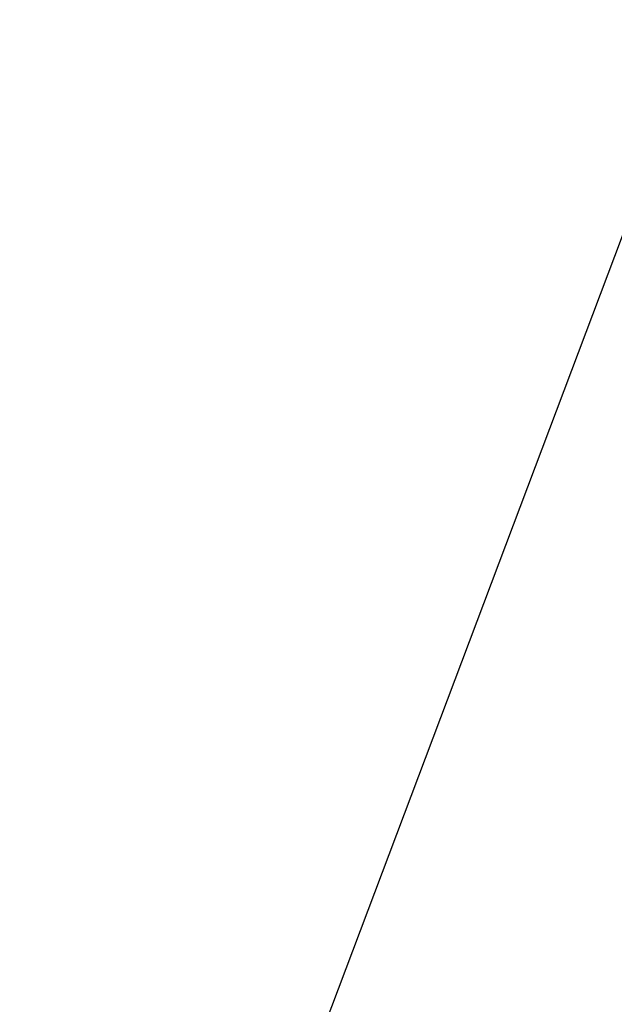
# Model space of a CAD drawing. Units: inches. Extents: x 3590 to 5167, y 65 to 1917.
# Tile 84 of 100: x 5051.5399 to 5051.6658, y 1788.6144 to 1788.8231. Entities that reach past the tile are written whole.
import ezdxf

# ---------------------------------------------------------------- set-up
doc = ezdxf.new("R2010")
doc.units = ezdxf.units.IN
for name, color, linetype, lineweight in [('A-ANNO-DIMS', 2, 'Continuous', 18), ('A-FLOR-PATT', 8, 'Continuous', 13), ('L-PLNT', 94, 'Continuous', 18)]:
    doc.layers.add(name, color=color, linetype=linetype, lineweight=lineweight)
doc.layers.add('DIENHOA', color=3, linetype='Continuous')
doc.styles.get("Standard").update_dxf_attribs({"font": 'arial.ttf'})
doc.dimstyles.new('ISO-25', dxfattribs={"dimtxt": 9, "dimasz": 2.5, "dimexe": 1.25, "dimexo": 0.625, "dimtad": 1, "dimdec": 1, "dimlunit": 3, "dimtxsty": 'Standard', "dimcen": 2.5, "dimadec": 0, "dimazin": 0, "dimtfac": 1, "dimtdec": 1, "dimtmove": 0, "dimatfit": 3, "dimfxl": 1, "dimarcsym": 0})

# ---------------------------------------------------------------- blocks, each defined once
blk = doc.blocks.new('Cay03_mb')
at = {"layer": 'DIENHOA'}
blk.add_lwpolyline([(23.6875, -5.4391), (19.839, 92.9868), (20.2832, 176.9678), (25.016, 248.5475), (34.0335, 309.7692), (47.3314, 362.6766), (64.9059, 409.3131), (86.7528, 451.7223), (112.868, 491.9476)], dxfattribs=at)
blk = doc.blocks.new('*D323')
at = {"layer": 'A-ANNO-DIMS', "color": 0, "lineweight": -2, "transparency": 16777216}
for p, q in [((5069.17227, 1795.21603), (5069.17227, 1874.95034)), ((5065.43703, 1795.21603), (5070.42227, 1795.21603)), ((5069.17227, 1769.30924), (5069.17227, 1792.71603)), ((5065.43703, 1766.80924), (5070.42227, 1766.80924))]:
    blk.add_line(p, q, dxfattribs=at)
at = {"layer": 'A-ANNO-DIMS', "color": 0, "transparency": 16777216}
for points in [[(5068.75561, 1792.71603), (5069.58894, 1792.71603), (5069.17227, 1795.21603)], [(5068.75561, 1769.30924), (5069.58894, 1769.30924), (5069.17227, 1766.80924)]]:
    blk.add_solid(points, dxfattribs=at)
at = {"layer": 'Defpoints', "color": 0, "transparency": 16777216}
for p in [(5064.81203, 1795.21603), (5069.17227, 1795.21603), (5064.81203, 1766.80924)]:
    blk.add_point(p, dxfattribs=at)
at = {"layer": 'A-ANNO-DIMS', "color": 0, "transparency": 16777216, "insert": (5063.89379, 1836.33318), "char_height": 9, "attachment_point": 5, "rotation": 90}
blk.add_mtext('2\'-4 1/2" TYP.', dxfattribs=at)

msp = doc.modelspace()

# ---------------------------------------------------------------- hatches: boundary and pattern name
at = {"layer": 'A-FLOR-PATT', "transparency": 33554687}
h = msp.add_hatch(dxfattribs=at)
h.set_pattern_fill('AR-HBONE', color=256, scale=0.2)
h.set_pattern_definition([(45, (-588.972, 0), (0, 28.73682), [60.96, -20.32]), (135, (-574.604, 14.368), (3e-15, 28.73682), [60.96, -20.32])])
h.paths.add_polyline_path([(5071.27403, 1796.99898), (4933.27403, 1796.99898), (4933.27403, 1753.99898), (4962.77403, 1753.99898, -0.414214), (4928.77403, 1719.99898), (4933.27403, 1718.99898), (4933.27403, 1334.99898), (5071.27403, 1334.99898)])
h.paths.add_polyline_path([(4951.78002, 1521.0767), (4951.7151, 1521.0404), (4951.56345, 1520.89532)], flags=16)
h.paths.add_polyline_path([(4952.267, 1521.37645), (4952.1977, 1521.37111), (4952.19823, 1521.35558)], flags=0)
h.paths.add_polyline_path([(4967.05076, 1529.72832), (4965.23122, 1528.69444), (4963.41109, 1527.71401), (4961.75649, 1526.85081), (4963.58887, 1527.44938), (4964.03555, 1527.47802), (4962.9755, 1527.24902), (4961.76022, 1526.85203), (4959.79219, 1525.83406), (4958.00498, 1524.89483), (4956.24031, 1523.92961), (4954.50395, 1522.91854), (4954.1294, 1522.68163), (4953.36051, 1521.99688), (4953.36558, 1521.99754), (4953.605, 1522.06367), (4955.10605, 1522.76083), (4956.92108, 1523.43405), (4958.67784, 1523.91513), (4960.35834, 1524.20036), (4961.94456, 1524.28606), (4964.17144, 1524.10849), (4965.95752, 1523.30903), (4963.86273, 1522.97565), (4965.18742, 1522.49898), (4963.36614, 1522.49715), (4961.54526, 1522.48682), (4959.76359, 1522.46077), (4958.30414, 1522.4188), (4957.97356, 1522.38829), (4956.30692, 1522.2324), (4954.71821, 1522.07143), (4953.25077, 1521.89915), (4953.52509, 1521.62277), (4954.33087, 1521.37883), (4956.24263, 1521.22987), (4958.03913, 1520.92952), (4959.68424, 1520.48339), (4961.16007, 1519.89569), (4963.10699, 1518.80022), (4964.39286, 1517.32518), (4962.97306, 1517.72596), (4964.55841, 1516.66059), (4965.40664, 1515.70779), (4963.50733, 1516.32179), (4961.67995, 1517.0051), (4959.93478, 1517.74489), (4958.2821, 1518.52833), (4956.73216, 1519.34257), (4955.29527, 1520.17478), (4954.67155, 1520.57237), (4954.51279, 1520.6271), (4955.65848, 1519.31837), (4956.70263, 1517.98232), (4957.64403, 1516.64663), (4958.48545, 1515.33439), (4959.54998, 1513.52398), (4960.43768, 1511.76936), (4958.84107, 1513.6196), (4957.45175, 1515.3249), (4955.8186, 1517.45855), (4956.66537, 1515.44764), (4957.11109, 1513.92292), (4957.44681, 1511.71434), (4957.07641, 1509.79288), (4956.53757, 1511.1103), (4955.99231, 1512.56892), (4955.44448, 1514.12509), (4954.89794, 1515.73518), (4954.35653, 1517.35553), (4953.82412, 1518.94251), (4953.30455, 1520.45247), (4953.06452, 1521.11563), (4952.97143, 1521.14607), (4952.94932, 1521.08646), (4952.72981, 1520.19905), (4953.3698, 1518.02364), (4953.75708, 1516.37279), (4954.05124, 1514.76538), (4954.26449, 1513.22121), (4954.47124, 1511.13121), (4954.4971, 1510.40174), (4954.40903, 1511.76006), (4954.26449, 1513.22121), (4954.05124, 1514.76538), (4953.75708, 1516.37279), (4953.3698, 1518.02364), (4952.87718, 1519.69813), (4952.7161, 1520.1412), (4952.53301, 1519.05871), (4952.37428, 1517.78881), (4952.21925, 1516.31167), (4952.04598, 1514.59986), (4951.83253, 1512.62598), (4951.55697, 1510.36259), (4951.20331, 1512.16818), (4950.85168, 1514.33931), (4950.98529, 1516.37594), (4951.6596, 1518.28625), (4952.59261, 1520.48085), (4952.35664, 1521.1299), (4951.85502, 1520.32753), (4950.83901, 1518.90828), (4949.77675, 1517.58658), (4948.91554, 1516.61731), (4948.11099, 1515.2561), (4947.0891, 1513.55389), (4945.88937, 1511.61495), (4946.32587, 1513.40232), (4946.5624, 1514.24913), (4945.52771, 1513.32668), (4944.58105, 1512.53126), (4946.01774, 1514.50825), (4947.2044, 1516.04763), (4947.89331, 1517.31331), (4949.30686, 1518.76446), (4950.41417, 1519.76716), (4950.45131, 1519.80628), (4952.267, 1521.37645), (4951.64457, 1521.49317), (4950.40371, 1521.17954), (4948.04447, 1520.35868), (4946.11863, 1519.45198), (4944.57182, 1518.47484), (4943.34962, 1517.44265), (4941.99695, 1515.91971), (4941.66146, 1515.27475), (4942.81332, 1516.98973), (4944.57182, 1518.47484), (4946.11863, 1519.45198), (4948.04447, 1520.35868), (4950.40371, 1521.17954), (4951.64457, 1521.49317), (4949.64678, 1521.86781), (4948.59979, 1521.75633), (4947.12629, 1521.5699), (4945.42015, 1521.34763), (4943.44969, 1521.10462), (4941.18319, 1520.85596), (4942.86028, 1521.61265), (4943.87308, 1522.03014), (4942.95216, 1521.9093), (4941.40968, 1521.48512), (4939.54287, 1520.67019), (4938.96775, 1520.2255), (4940.73284, 1521.29899), (4942.95216, 1521.9093), (4943.70184, 1522.00767), (4945.89419, 1522.69998), (4947.56488, 1522.71399), (4948.92086, 1522.56573), (4951.13144, 1522.18271), (4950.97062, 1522.2969), (4948.12924, 1523.00563), (4946.03496, 1523.70671), (4944.23235, 1524.52143), (4942.70692, 1525.46111), (4941.44419, 1526.53707), (4940.42968, 1527.76062), (4939.6489, 1529.14306), (4941.42091, 1528.12232), (4943.14742, 1527.13248), (4944.84093, 1526.17457), (4946.51394, 1525.24959), (4948.17893, 1524.35855), (4948.36457, 1524.26336), (4946.47531, 1526.04459), (4945.18083, 1527.54042), (4944.19039, 1529.03339), (4943.49559, 1530.53985), (4943.27808, 1531.3597), (4942.49849, 1531.91903), (4943.11353, 1531.76249), (4942.95927, 1533.6586), (4944.13953, 1531.9886), (4944.61171, 1531.32339), (4946.20163, 1530.46341), (4947.48567, 1529.50925), (4948.79027, 1528.22649), (4950.36754, 1526.23746), (4949.48547, 1528.15549), (4948.85128, 1530.12254), (4948.49054, 1532.04127), (4948.38105, 1533.91822), (4948.50062, 1535.7599), (4948.82704, 1537.57284), (4949.41803, 1535.56526), (4949.95684, 1533.56932), (4950.46414, 1531.5861), (4950.96058, 1529.6167), (4951.3911, 1527.95448), (4951.72352, 1530.68689), (4952.20106, 1532.57994), (4952.88914, 1534.32964), (4953.77035, 1535.95123), (4954.82726, 1537.45995), (4954.52145, 1535.38966), (4954.27314, 1533.93684), (4955.57999, 1535.6627), (4956.74758, 1536.73859), (4956.15852, 1534.78029), (4955.58917, 1532.87334), (4955.04336, 1531.00581), (4954.52493, 1529.16576), (4954.03771, 1527.34127), (4953.63833, 1525.73298), (4953.61143, 1525.58564), (4953.39805, 1524.16565), (4953.38219, 1524.00887), (4954.06955, 1525.47563), (4954.91212, 1527.02173), (4956.13627, 1528.89351), (4957.84668, 1530.57701), (4959.37601, 1531.54014), (4958.25596, 1530.10398), (4957.14284, 1528.66291), (4956.06626, 1527.24305), (4955.05579, 1525.87054), (4954.14104, 1524.57149), (4953.35159, 1523.37204), (4953.31079, 1523.30299), (4953.27253, 1522.92478), (4953.26102, 1522.38213), (4954.1031, 1523.37273), (4954.63005, 1524.28376), (4955.96149, 1526.35767), (4957.23002, 1528.12969), (4958.42057, 1529.60864), (4960.03671, 1531.36792), (4961.3736, 1532.3752), (4962.1015, 1532.77), (4961.06994, 1531.06113), (4959.98733, 1529.43811), (4958.86851, 1527.90803), (4958.15046, 1527.00742), (4959.80291, 1528.00314), (4961.58854, 1528.79257), (4963.39087, 1529.32783), (4965.21118, 1529.63205)], flags=16)
h.paths.add_polyline_path([(4962.94387, 1523.18187), (4961.10714, 1523.42192), (4960.39205, 1523.36158), (4962.34964, 1523.33061)], flags=0)
h.paths.add_polyline_path([(5049.54129, 1584.55089), (5049.47636, 1584.51458), (5049.32471, 1584.3695)], flags=16)
h.paths.add_polyline_path([(5050.02827, 1584.85063), (5049.95897, 1584.84529), (5049.95949, 1584.82976)], flags=0)
h.paths.add_polyline_path([(5042.33308, 1581.94902), (5043.8799, 1582.92616), (5045.80573, 1583.83286), (5048.16498, 1584.65372), (5049.40583, 1584.96736), (5047.40804, 1585.34199), (5046.36106, 1585.23052), (5044.88755, 1585.04408), (5043.18142, 1584.82181), (5041.21095, 1584.5788), (5038.94446, 1584.33014), (5040.62155, 1585.08683), (5041.63434, 1585.50432), (5040.71343, 1585.38348), (5039.17095, 1584.9593), (5037.30414, 1584.14438), (5036.72901, 1583.69969), (5038.4941, 1584.77317), (5040.71343, 1585.38348), (5041.4631, 1585.48185), (5043.65545, 1586.17416), (5045.32615, 1586.18818), (5046.68212, 1586.03992), (5048.8927, 1585.6569), (5048.73188, 1585.77108), (5045.89051, 1586.47981), (5043.79622, 1587.18089), (5041.99361, 1587.99561), (5040.46818, 1588.9353), (5039.20546, 1590.01125), (5038.19095, 1591.2348), (5037.41016, 1592.61725), (5039.18217, 1591.5965), (5040.90868, 1590.60667), (5042.6022, 1589.64876), (5044.2752, 1588.72378), (5045.94019, 1587.83274), (5046.12584, 1587.73754), (5044.23658, 1589.51878), (5042.9421, 1591.01461), (5041.95166, 1592.50757), (5041.25685, 1594.01403), (5041.03935, 1594.83388), (5040.25976, 1595.39321), (5040.8748, 1595.23667), (5040.72054, 1597.13279), (5041.9008, 1595.46278), (5042.37297, 1594.79758), (5043.96289, 1593.93759), (5045.24694, 1592.98344), (5046.55153, 1591.70068), (5048.12881, 1589.71164), (5047.24673, 1591.62967), (5046.61254, 1593.59672), (5046.2518, 1595.51546), (5046.14232, 1597.3924), (5046.26189, 1599.23408), (5046.5883, 1601.04703), (5047.17929, 1599.03944), (5047.71811, 1597.0435), (5048.22541, 1595.06028), (5048.72184, 1593.09089), (5049.15237, 1591.42866), (5049.48478, 1594.16107), (5049.96233, 1596.05412), (5050.65041, 1597.80382), (5051.53161, 1599.42541), (5052.58852, 1600.93414), (5052.28271, 1598.86384), (5052.03441, 1597.41102), (5053.34126, 1599.13689), (5054.50884, 1600.21277), (5053.91979, 1598.25447), (5053.35044, 1596.34752), (5052.80463, 1594.47999), (5052.2862, 1592.63995), (5051.79898, 1590.81546), (5051.39959, 1589.20716), (5051.3727, 1589.05983), (5051.15931, 1587.63984), (5051.14346, 1587.48305), (5051.83082, 1588.94982), (5052.67339, 1590.49592), (5053.89754, 1592.3677), (5055.60794, 1594.05119), (5057.13728, 1595.01432), (5056.01722, 1593.57817), (5054.90411, 1592.1371), (5053.82752, 1590.71724), (5052.81705, 1589.34472), (5051.9023, 1588.04567), (5051.11286, 1586.84622), (5051.07205, 1586.77718), (5051.03379, 1586.39896), (5051.02228, 1585.85631), (5051.86437, 1586.84692), (5052.39131, 1587.75794), (5053.72275, 1589.83185), (5054.99128, 1591.60387), (5056.18183, 1593.08282), (5057.79798, 1594.84211), (5059.13486, 1595.84938), (5059.86276, 1596.24419), (5058.83121, 1594.53531), (5057.7486, 1592.9123), (5056.62978, 1591.38221), (5055.91173, 1590.4816), (5057.56418, 1591.47732), (5059.34981, 1592.26675), (5061.15214, 1592.80202), (5062.97245, 1593.10624), (5064.81203, 1593.20251), (5062.99248, 1592.16863), (5061.17235, 1591.18819), (5059.51775, 1590.325), (5061.35014, 1590.92356), (5061.79682, 1590.95221), (5060.73676, 1590.7232), (5059.52148, 1590.32622), (5057.55345, 1589.30825), (5055.76625, 1588.36901), (5054.00157, 1587.40379), (5052.26521, 1586.39273), (5051.89067, 1586.15581), (5051.12177, 1585.47106), (5051.12684, 1585.47172), (5051.36627, 1585.53786), (5052.86732, 1586.23502), (5054.68234, 1586.90824), (5056.4391, 1587.38931), (5058.1196, 1587.67454), (5059.70582, 1587.76024), (5061.93271, 1587.58268), (5063.71878, 1586.78321), (5061.62399, 1586.44983), (5062.94869, 1585.97317), (5061.12741, 1585.97133), (5059.30653, 1585.961), (5057.52486, 1585.93496), (5056.06541, 1585.89299), (5055.73482, 1585.86247), (5054.06819, 1585.70658), (5052.47947, 1585.54561), (5051.01204, 1585.37333), (5051.28635, 1585.09695), (5052.09214, 1584.85301), (5054.00389, 1584.70406), (5055.8004, 1584.4037), (5057.44551, 1583.95757), (5058.92133, 1583.36987), (5060.86825, 1582.27441), (5062.15413, 1580.79937), (5060.73433, 1581.20015), (5062.31967, 1580.13477), (5063.1679, 1579.18198), (5061.2686, 1579.79597), (5059.44122, 1580.47928), (5057.69605, 1581.21908), (5056.04336, 1582.00251), (5054.49343, 1582.81675), (5053.05653, 1583.64897), (5052.43281, 1584.04656), (5052.27405, 1584.10128), (5053.41974, 1582.79255), (5054.4639, 1581.4565), (5055.40529, 1580.12081), (5056.24672, 1578.80858), (5057.31125, 1576.99816), (5058.19895, 1575.24354), (5056.60234, 1577.09378), (5055.21301, 1578.79908), (5053.57987, 1580.93274), (5054.42664, 1578.92183), (5054.87235, 1577.3971), (5055.20808, 1575.18852), (5054.83767, 1573.26706), (5054.29883, 1574.58448), (5053.75357, 1576.0431), (5053.20575, 1577.59927), (5052.6592, 1579.20936), (5052.1178, 1580.82971), (5051.58538, 1582.41669), (5051.06582, 1583.92666), (5050.82578, 1584.58981), (5050.7327, 1584.62025), (5050.71058, 1584.56064), (5050.49108, 1583.67323), (5051.13107, 1581.49782), (5051.51835, 1579.84698), (5051.8125, 1578.23957), (5052.02575, 1576.69539), (5052.23251, 1574.6054), (5052.25836, 1573.87593), (5052.1703, 1575.23424), (5052.02575, 1576.69539), (5051.8125, 1578.23957), (5051.51835, 1579.84698), (5051.13107, 1581.49782), (5050.63844, 1583.17231), (5050.47736, 1583.61538), (5050.29428, 1582.53289), (5050.13554, 1581.26299), (5049.98051, 1579.78585), (5049.80724, 1578.07405), (5049.59379, 1576.10016), (5049.31823, 1573.83678), (5048.96458, 1575.64237), (5048.61294, 1577.8135), (5048.74656, 1579.85012), (5049.42086, 1581.76043), (5050.35388, 1583.95503), (5050.1179, 1584.60408), (5049.61629, 1583.80172), (5048.60027, 1582.38246), (5047.53801, 1581.06076), (5046.67681, 1580.09149), (5045.87225, 1578.73029), (5044.85036, 1577.02808), (5043.65063, 1575.08913), (5044.08713, 1576.8765), (5044.32366, 1577.72331), (5043.28898, 1576.80086), (5042.34232, 1576.00545), (5043.779, 1577.98243), (5044.96566, 1579.52182), (5045.65457, 1580.78749), (5047.06813, 1582.23865), (5048.17543, 1583.24134), (5048.21258, 1583.28047), (5050.02827, 1584.85063), (5049.40583, 1584.96736), (5048.16498, 1584.65372), (5045.80573, 1583.83286), (5043.8799, 1582.92616), (5042.33308, 1581.94902), (5041.11088, 1580.91684), (5039.75821, 1579.39389), (5039.42272, 1578.74894), (5040.57458, 1580.46391)], flags=16)
h.paths.add_polyline_path([(4954.79872, 1533.12029), (4954.26249, 1532.07935), (4953.83112, 1530.93464), (4953.50472, 1529.63602), (4953.28338, 1528.13331), (4953.16721, 1526.37637), (4953.15631, 1524.31504), (4953.27669, 1521.23629), (4952.80168, 1521.84177), (4951.55695, 1521.99789), (4950.97575, 1521.9613), (4952.66059, 1521.94097), (4952.80168, 1521.84177), (4953.15249, 1523.59258), (4953.16721, 1526.37637), (4953.28338, 1528.13331), (4953.60929, 1530.34598), (4954.45558, 1532.59174)], flags=0)
h.paths.add_polyline_path([(5050.56294, 1585.31596), (5049.31822, 1585.47208), (5048.73702, 1585.43548), (5050.42186, 1585.41516), (5050.56294, 1585.31596), (5050.91375, 1587.06676), (5050.92848, 1589.85056), (5051.04465, 1591.6075), (5051.37055, 1593.82017), (5052.21684, 1596.06593), (5052.55999, 1596.59447), (5052.02375, 1595.55353), (5051.59238, 1594.40883), (5051.26598, 1593.1102), (5051.04465, 1591.6075), (5050.92848, 1589.85056), (5050.91757, 1587.78922), (5051.03795, 1584.71048)], flags=0)
h.paths.add_polyline_path([(5058.15332, 1586.83576), (5060.11091, 1586.80479), (5060.70514, 1586.65605), (5058.8684, 1586.8961)], flags=0)
h.paths.add_polyline_path([(5049.54129, 1430.93611), (5049.47636, 1430.8998), (5049.32471, 1430.75472)], flags=16)
h.paths.add_polyline_path([(5050.02827, 1431.23585), (5049.95897, 1431.23051), (5049.95949, 1431.21498)], flags=0)
h.paths.add_polyline_path([(5046.5883, 1447.43225), (5047.17929, 1445.42467), (5047.71811, 1443.42872), (5048.22541, 1441.4455), (5048.72184, 1439.47611), (5049.15237, 1437.81388), (5049.48478, 1440.5463), (5049.96233, 1442.43934), (5050.65041, 1444.18904), (5051.53161, 1445.81063), (5052.58852, 1447.31936), (5052.28271, 1445.24906), (5052.03441, 1443.79624), (5053.34126, 1445.52211), (5054.50884, 1446.59799), (5053.91979, 1444.63969), (5053.35044, 1442.73274), (5052.80463, 1440.86521), (5052.2862, 1439.02517), (5051.79898, 1437.20068), (5051.39959, 1435.59238), (5051.3727, 1435.44505), (5051.15931, 1434.02506), (5051.14346, 1433.86828), (5051.83082, 1435.33504), (5052.67339, 1436.88114), (5053.89754, 1438.75292), (5055.60794, 1440.43641), (5057.13728, 1441.39954), (5056.01722, 1439.96339), (5054.90411, 1438.52232), (5053.82752, 1437.10246), (5052.81705, 1435.72994), (5051.9023, 1434.4309), (5051.11286, 1433.23145), (5051.07205, 1433.1624), (5051.03379, 1432.78418), (5051.02228, 1432.24153), (5051.86437, 1433.23214), (5052.39131, 1434.14316), (5053.72275, 1436.21707), (5054.99128, 1437.98909), (5056.18183, 1439.46805), (5057.79798, 1441.22733), (5059.13486, 1442.23461), (5059.86276, 1442.62941), (5058.83121, 1440.92053), (5057.7486, 1439.29752), (5056.62978, 1437.76743), (5055.91173, 1436.86682), (5057.56418, 1437.86255), (5059.34981, 1438.65197), (5061.15214, 1439.18724), (5062.97245, 1439.49146), (5064.81203, 1439.58773), (5062.99248, 1438.55385), (5061.17235, 1437.57342), (5059.51775, 1436.71022), (5061.35014, 1437.30879), (5061.79682, 1437.33743), (5060.73676, 1437.10842), (5059.52148, 1436.71144), (5057.55345, 1435.69347), (5055.76625, 1434.75423), (5054.00157, 1433.78901), (5052.26521, 1432.77795), (5051.89067, 1432.54103), (5051.12177, 1431.85628), (5051.12684, 1431.85694), (5051.36627, 1431.92308), (5052.86732, 1432.62024), (5054.68234, 1433.29346), (5056.4391, 1433.77453), (5058.1196, 1434.05976), (5059.70582, 1434.14546), (5061.93271, 1433.9679), (5063.71878, 1433.16843), (5061.62399, 1432.83505), (5062.94869, 1432.35839), (5061.12741, 1432.35655), (5059.30653, 1432.34623), (5057.52486, 1432.32018), (5056.06541, 1432.27821), (5055.73482, 1432.24769), (5054.06819, 1432.09181), (5052.47947, 1431.93083), (5051.01204, 1431.75856), (5051.28635, 1431.48218), (5052.09214, 1431.23823), (5054.00389, 1431.08928), (5055.8004, 1430.78892), (5057.44551, 1430.34279), (5058.92133, 1429.75509), (5060.86825, 1428.65963), (5062.15413, 1427.18459), (5060.73433, 1427.58537), (5062.31967, 1426.52), (5063.1679, 1425.5672), (5061.2686, 1426.18119), (5059.44122, 1426.86451), (5057.69605, 1427.6043), (5056.04336, 1428.38773), (5054.49343, 1429.20197), (5053.05653, 1430.03419), (5052.43281, 1430.43178), (5052.27405, 1430.48651), (5053.41974, 1429.17777), (5054.4639, 1427.84172), (5055.40529, 1426.50603), (5056.24672, 1425.1938), (5057.31125, 1423.38338), (5058.19895, 1421.62877), (5056.60234, 1423.479), (5055.21301, 1425.1843), (5053.57987, 1427.31796), (5054.42664, 1425.30705), (5054.87235, 1423.78233), (5055.20808, 1421.57374), (5054.83767, 1419.65228), (5054.29883, 1420.9697), (5053.75357, 1422.42832), (5053.20575, 1423.9845), (5052.6592, 1425.59458), (5052.1178, 1427.21493), (5051.58538, 1428.80191), (5051.06582, 1430.31188), (5050.82578, 1430.97503), (5050.7327, 1431.00547), (5050.71058, 1430.94586), (5050.49108, 1430.05845), (5051.13107, 1427.88305), (5051.51835, 1426.2322), (5051.8125, 1424.62479), (5052.02575, 1423.08061), (5052.23251, 1420.99062), (5052.25836, 1420.26115), (5052.1703, 1421.61947), (5052.02575, 1423.08061), (5051.8125, 1424.62479), (5051.51835, 1426.2322), (5051.13107, 1427.88305), (5050.63844, 1429.55753), (5050.47736, 1430.0006), (5050.29428, 1428.91811), (5050.13554, 1427.64821), (5049.98051, 1426.17107), (5049.80724, 1424.45927), (5049.59379, 1422.48539), (5049.31823, 1420.222), (5048.96458, 1422.02759), (5048.61294, 1424.19872), (5048.74656, 1426.23534), (5049.42086, 1428.14565), (5050.35388, 1430.34025), (5050.1179, 1430.98931), (5049.61629, 1430.18694), (5048.60027, 1428.76768), (5047.53801, 1427.44598), (5046.67681, 1426.47671), (5045.87225, 1425.11551), (5044.85036, 1423.4133), (5043.65063, 1421.47435), (5044.08713, 1423.26172), (5044.32366, 1424.10854), (5043.28898, 1423.18608), (5042.34232, 1422.39067), (5043.779, 1424.36765), (5044.96566, 1425.90704), (5045.65457, 1427.17272), (5047.06813, 1428.62387), (5048.17543, 1429.62657), (5048.21258, 1429.66569), (5050.02827, 1431.23585), (5049.40583, 1431.35258), (5048.16498, 1431.03894), (5045.80573, 1430.21809), (5043.8799, 1429.31139), (5042.33308, 1428.33424), (5041.11088, 1427.30206), (5039.75821, 1425.77911), (5039.42272, 1425.13416), (5040.57458, 1426.84914), (5042.33308, 1428.33424), (5043.8799, 1429.31139), (5045.80573, 1430.21809), (5048.16498, 1431.03894), (5049.40583, 1431.35258), (5047.40804, 1431.72722), (5046.36106, 1431.61574), (5044.88755, 1431.42931), (5043.18142, 1431.20704), (5041.21095, 1430.96402), (5038.94446, 1430.71536), (5040.62155, 1431.47205), (5041.63434, 1431.88954), (5040.71343, 1431.76871), (5039.17095, 1431.34453), (5037.30414, 1430.5296), (5036.72901, 1430.08491), (5038.4941, 1431.1584), (5040.71343, 1431.76871), (5041.4631, 1431.86707), (5043.65545, 1432.55939), (5045.32615, 1432.5734), (5046.68212, 1432.42514), (5048.8927, 1432.04212), (5048.73188, 1432.1563), (5045.89051, 1432.86503), (5043.79622, 1433.56611), (5041.99361, 1434.38083), (5040.46818, 1435.32052), (5039.20546, 1436.39648), (5038.19095, 1437.62002), (5037.41016, 1439.00247), (5039.18217, 1437.98172), (5040.90868, 1436.99189), (5042.6022, 1436.03398), (5044.2752, 1435.109), (5045.94019, 1434.21796), (5046.12584, 1434.12276), (5044.23658, 1435.904), (5042.9421, 1437.39983), (5041.95166, 1438.8928), (5041.25685, 1440.39925), (5041.03935, 1441.2191), (5040.25976, 1441.77844), (5040.8748, 1441.62189), (5040.72054, 1443.51801), (5041.9008, 1441.848), (5042.37297, 1441.1828), (5043.96289, 1440.32282), (5045.24694, 1439.36866), (5046.55153, 1438.0859), (5048.12881, 1436.09686), (5047.24673, 1438.01489), (5046.61254, 1439.98195), (5046.2518, 1441.90068), (5046.14232, 1443.77762), (5046.26189, 1445.6193)], flags=16)
h.paths.add_polyline_path([(5052.38176, 1444.25496), (5051.62263, 1442.77987), (5052.02375, 1441.93875), (5052.55999, 1442.9797)], flags=0)
h.paths.add_polyline_path([(5050.56294, 1431.70118), (5049.31822, 1431.8573), (5048.73702, 1431.82071), (5050.42186, 1431.80038)], flags=0)
h.paths.add_polyline_path([(5058.15332, 1433.22098), (5060.11091, 1433.19001), (5060.70514, 1433.04127), (5058.8684, 1433.28132)], flags=0)
h.paths.add_polyline_path([(5049.54129, 1352.28535), (5049.47636, 1352.24904), (5049.32471, 1352.10396)], flags=16)
h.paths.add_polyline_path([(5050.02827, 1352.58509), (5049.95897, 1352.57975), (5049.95949, 1352.56422)], flags=0)
h.paths.add_polyline_path([(5046.5883, 1368.78149), (5047.17929, 1366.7739), (5047.71811, 1364.77796), (5048.22541, 1362.79474), (5048.72184, 1360.82534), (5049.15237, 1359.16312), (5049.48478, 1361.89553), (5049.96233, 1363.78858), (5050.65041, 1365.53828), (5051.53161, 1367.15987), (5052.58852, 1368.6686), (5052.28271, 1366.5983), (5052.03441, 1365.14548), (5053.34126, 1366.87135), (5054.50884, 1367.94723), (5053.91979, 1365.98893), (5053.35044, 1364.08198), (5052.80463, 1362.21445), (5052.2862, 1360.37441), (5051.79898, 1358.54992), (5051.39959, 1356.94162), (5051.3727, 1356.79428), (5051.15931, 1355.37429), (5051.14346, 1355.21751), (5051.83082, 1356.68428), (5052.67339, 1358.23037), (5053.89754, 1360.10216), (5055.60794, 1361.78565), (5057.13728, 1362.74878), (5056.01722, 1361.31262), (5054.90411, 1359.87155), (5053.82752, 1358.4517), (5052.81705, 1357.07918), (5051.9023, 1355.78013), (5051.11286, 1354.58068), (5051.07205, 1354.51164), (5051.03379, 1354.13342), (5051.02228, 1353.59077), (5051.86437, 1354.58137), (5052.39131, 1355.4924), (5053.72275, 1357.56631), (5054.99128, 1359.33833), (5056.18183, 1360.81728), (5057.79798, 1362.57656), (5059.13486, 1363.58384), (5059.86276, 1363.97864), (5058.83121, 1362.26977), (5057.7486, 1360.64675), (5056.62978, 1359.11667), (5055.91173, 1358.21606), (5057.56418, 1359.21178), (5059.34981, 1360.00121), (5061.15214, 1360.53648), (5062.97245, 1360.84069), (5064.81203, 1360.93697), (5062.99248, 1359.90308), (5061.17235, 1358.92265), (5059.51775, 1358.05946), (5061.35014, 1358.65802), (5061.79682, 1358.68666), (5060.73676, 1358.45766), (5059.52148, 1358.06068), (5057.55345, 1357.0427), (5055.76625, 1356.10347), (5054.00157, 1355.13825), (5052.26521, 1354.12718), (5051.89067, 1353.89027), (5051.12177, 1353.20552), (5051.12684, 1353.20618), (5051.36627, 1353.27231), (5052.86732, 1353.96947), (5054.68234, 1354.6427), (5056.4391, 1355.12377), (5058.1196, 1355.409), (5059.70582, 1355.4947), (5061.93271, 1355.31713), (5063.71878, 1354.51767), (5061.62399, 1354.18429), (5062.94869, 1353.70763), (5061.12741, 1353.70579), (5059.30653, 1353.69546), (5057.52486, 1353.66942), (5056.06541, 1353.62744), (5055.73482, 1353.59693), (5054.06819, 1353.44104), (5052.47947, 1353.28007), (5051.01204, 1353.10779), (5051.28635, 1352.83141), (5052.09214, 1352.58747), (5054.00389, 1352.43852), (5055.8004, 1352.13816), (5057.44551, 1351.69203), (5058.92133, 1351.10433), (5060.86825, 1350.00887), (5062.15413, 1348.53382), (5060.73433, 1348.9346), (5062.31967, 1347.86923), (5063.1679, 1346.91643), (5061.2686, 1347.53043), (5059.44122, 1348.21374), (5057.69605, 1348.95353), (5056.04336, 1349.73697), (5054.49343, 1350.55121), (5053.05653, 1351.38342), (5052.43281, 1351.78101), (5052.27405, 1351.83574), (5053.41974, 1350.52701), (5054.4639, 1349.19096), (5055.40529, 1347.85527), (5056.24672, 1346.54303), (5057.31125, 1344.73262), (5058.19895, 1342.978), (5056.60234, 1344.82824), (5055.21301, 1346.53354), (5053.57987, 1348.6672), (5054.42664, 1346.65629), (5054.87235, 1345.13156), (5055.20808, 1342.92298), (5054.83767, 1341.00152), (5054.29883, 1342.31894), (5053.75357, 1343.77756), (5053.20575, 1345.33373), (5052.6592, 1346.94382), (5052.1178, 1348.56417), (5051.58538, 1350.15115), (5051.06582, 1351.66111), (5050.82578, 1352.32427), (5050.7327, 1352.35471), (5050.71058, 1352.2951), (5050.49108, 1351.40769), (5051.13107, 1349.23228), (5051.51835, 1347.58144), (5051.8125, 1345.97403), (5052.02575, 1344.42985), (5052.23251, 1342.33986), (5052.25836, 1341.61039), (5052.1703, 1342.9687), (5052.02575, 1344.42985), (5051.8125, 1345.97403), (5051.51835, 1347.58144), (5051.13107, 1349.23228), (5050.63844, 1350.90677), (5050.47736, 1351.34984), (5050.29428, 1350.26735), (5050.13554, 1348.99745), (5049.98051, 1347.52031), (5049.80724, 1345.80851), (5049.59379, 1343.83462), (5049.31823, 1341.57124), (5048.96458, 1343.37683), (5048.61294, 1345.54796), (5048.74656, 1347.58458), (5049.42086, 1349.49489), (5050.35388, 1351.68949), (5050.1179, 1352.33854), (5049.61629, 1351.53617), (5048.60027, 1350.11692), (5047.53801, 1348.79522), (5046.67681, 1347.82595), (5045.87225, 1346.46475), (5044.85036, 1344.76253), (5043.65063, 1342.82359), (5044.08713, 1344.61096), (5044.32366, 1345.45777), (5043.28898, 1344.53532), (5042.34232, 1343.7399), (5043.779, 1345.71689), (5044.96566, 1347.25627), (5045.65457, 1348.52195), (5047.06813, 1349.9731), (5048.17543, 1350.9758), (5048.21258, 1351.01493), (5050.02827, 1352.58509), (5049.40583, 1352.70181), (5048.16498, 1352.38818), (5045.80573, 1351.56732), (5043.8799, 1350.66062), (5042.33308, 1349.68348), (5041.11088, 1348.65129), (5039.75821, 1347.12835), (5039.42272, 1346.4834), (5040.57458, 1348.19837), (5042.33308, 1349.68348), (5043.8799, 1350.66062), (5045.80573, 1351.56732), (5048.16498, 1352.38818), (5049.40583, 1352.70181), (5047.40804, 1353.07645), (5046.36106, 1352.96498), (5044.88755, 1352.77854), (5043.18142, 1352.55627), (5041.21095, 1352.31326), (5038.94446, 1352.0646), (5040.62155, 1352.82129), (5041.63434, 1353.23878), (5040.71343, 1353.11794), (5039.17095, 1352.69376), (5037.30414, 1351.87884), (5036.72901, 1351.43415), (5038.4941, 1352.50763), (5040.71343, 1353.11794), (5041.4631, 1353.21631), (5043.65545, 1353.90862), (5045.32615, 1353.92263), (5046.68212, 1353.77438), (5048.8927, 1353.39136), (5048.73188, 1353.50554), (5045.89051, 1354.21427), (5043.79622, 1354.91535), (5041.99361, 1355.73007), (5040.46818, 1356.66975), (5039.20546, 1357.74571), (5038.19095, 1358.96926), (5037.41016, 1360.35171), (5039.18217, 1359.33096), (5040.90868, 1358.34112), (5042.6022, 1357.38321), (5044.2752, 1356.45824), (5045.94019, 1355.5672), (5046.12584, 1355.472), (5044.23658, 1357.25323), (5042.9421, 1358.74906), (5041.95166, 1360.24203), (5041.25685, 1361.74849), (5041.03935, 1362.56834), (5040.25976, 1363.12767), (5040.8748, 1362.97113), (5040.72054, 1364.86725), (5041.9008, 1363.19724), (5042.37297, 1362.53203), (5043.96289, 1361.67205), (5045.24694, 1360.7179), (5046.55153, 1359.43513), (5048.12881, 1357.4461), (5047.24673, 1359.36413), (5046.61254, 1361.33118), (5046.2518, 1363.24992), (5046.14232, 1365.12686), (5046.26189, 1366.96854)], flags=16)
h.paths.add_polyline_path([(5052.38176, 1365.6042), (5051.62263, 1364.12911), (5052.02375, 1363.28799), (5052.55999, 1364.32893)], flags=0)
h.paths.add_polyline_path([(4951.78002, 1698.04081), (4951.7151, 1698.0045), (4951.56345, 1697.85942)], flags=16)
h.paths.add_polyline_path([(4952.267, 1698.34055), (4952.1977, 1698.33521), (4952.19823, 1698.31968)], flags=0)
h.paths.add_polyline_path([(4957.07641, 1686.75698), (4956.53757, 1688.0744), (4955.99231, 1689.53302), (4955.44448, 1691.08919), (4954.89794, 1692.69928), (4954.35653, 1694.31963), (4953.82412, 1695.90661), (4953.30455, 1697.41658), (4953.06452, 1698.07973), (4952.97143, 1698.11017), (4952.94932, 1698.05056), (4952.72981, 1697.16315), (4953.3698, 1694.98774), (4953.75708, 1693.3369), (4954.05124, 1691.72949), (4954.26449, 1690.18531), (4954.47124, 1688.09532), (4954.4971, 1687.36585), (4954.40903, 1688.72416), (4954.26449, 1690.18531), (4954.05124, 1691.72949), (4953.75708, 1693.3369), (4953.3698, 1694.98774), (4952.87718, 1696.66223), (4952.7161, 1697.1053), (4952.53301, 1696.02281), (4952.37428, 1694.75291), (4952.21925, 1693.27577), (4952.04598, 1691.56397), (4951.83253, 1689.59008), (4951.55697, 1687.3267), (4951.20331, 1689.13229), (4950.85168, 1691.30342), (4950.98529, 1693.34004), (4951.6596, 1695.25035), (4952.59261, 1697.44495), (4952.35664, 1698.09401), (4951.85502, 1697.29164), (4950.83901, 1695.87238), (4949.77675, 1694.55068), (4948.91554, 1693.58141), (4948.11099, 1692.22021), (4947.0891, 1690.518), (4945.88937, 1688.57905), (4946.32587, 1690.36642), (4946.5624, 1691.21323), (4945.52771, 1690.29078), (4944.58105, 1689.49537), (4946.01774, 1691.47235), (4947.2044, 1693.01174), (4947.89331, 1694.27741), (4949.30686, 1695.72857), (4950.41417, 1696.73127), (4950.45131, 1696.77039), (4952.267, 1698.34055), (4951.64457, 1698.45728), (4950.40371, 1698.14364), (4948.04447, 1697.32278), (4946.11863, 1696.41608), (4944.57182, 1695.43894), (4943.34962, 1694.40676), (4941.99695, 1692.88381), (4941.66146, 1692.23886), (4942.81332, 1693.95383), (4944.57182, 1695.43894), (4946.11863, 1696.41608), (4948.04447, 1697.32278), (4950.40371, 1698.14364), (4951.64457, 1698.45728), (4949.64678, 1698.83191), (4948.59979, 1698.72044), (4947.12629, 1698.53401), (4945.42015, 1698.31174), (4943.44969, 1698.06872), (4941.18319, 1697.82006), (4942.86028, 1698.57675), (4943.87308, 1698.99424), (4942.95216, 1698.8734), (4941.40968, 1698.44922), (4939.54287, 1697.6343), (4938.96775, 1697.18961), (4940.73284, 1698.26309), (4942.95216, 1698.8734), (4943.70184, 1698.97177), (4945.89419, 1699.66409), (4947.56488, 1699.6781), (4948.92086, 1699.52984), (4951.13144, 1699.14682), (4950.97062, 1699.261), (4948.12924, 1699.96973), (4946.03496, 1700.67081), (4944.23235, 1701.48553), (4942.70692, 1702.42522), (4941.44419, 1703.50117), (4940.42968, 1704.72472), (4939.6489, 1706.10717), (4941.42091, 1705.08642), (4943.14742, 1704.09659), (4944.84093, 1703.13868), (4946.51394, 1702.2137), (4948.17893, 1701.32266), (4948.36457, 1701.22746), (4946.47531, 1703.0087), (4945.18083, 1704.50453), (4944.19039, 1705.9975), (4943.49559, 1707.50395), (4943.27808, 1708.3238), (4942.49849, 1708.88314), (4943.11353, 1708.72659), (4942.95927, 1710.62271), (4944.13953, 1708.9527), (4944.61171, 1708.2875), (4946.20163, 1707.42751), (4947.48567, 1706.47336), (4948.79027, 1705.1906), (4950.36754, 1703.20156), (4949.48547, 1705.11959), (4948.85128, 1707.08664), (4948.49054, 1709.00538), (4948.38105, 1710.88232), (4948.50062, 1712.724), (4948.82704, 1714.53695), (4949.41803, 1712.52937), (4949.95684, 1710.53342), (4950.46414, 1708.5502), (4950.96058, 1706.58081), (4951.3911, 1704.91858), (4951.72352, 1707.65099), (4952.20106, 1709.54404), (4952.88914, 1711.29374), (4953.77035, 1712.91533), (4954.82726, 1714.42406), (4954.52145, 1712.35376), (4954.27314, 1710.90094), (4955.57999, 1712.62681), (4956.74758, 1713.70269), (4956.15852, 1711.74439), (4955.58917, 1709.83744), (4955.04336, 1707.96991), (4954.52493, 1706.12987), (4954.03771, 1704.30538), (4953.63833, 1702.69708), (4953.61143, 1702.54975), (4953.39805, 1701.12976), (4953.38219, 1700.97297), (4954.06955, 1702.43974), (4954.91212, 1703.98584), (4956.13627, 1705.85762), (4957.84668, 1707.54111), (4959.37601, 1708.50424), (4958.25596, 1707.06809), (4957.14284, 1705.62702), (4956.06626, 1704.20716), (4955.05579, 1702.83464), (4954.14104, 1701.53559), (4953.35159, 1700.33614), (4953.31079, 1700.2671), (4953.27253, 1699.88888), (4953.26102, 1699.34623), (4954.1031, 1700.33684), (4954.63005, 1701.24786), (4955.96149, 1703.32177), (4957.23002, 1705.09379), (4958.42057, 1706.57274), (4960.03671, 1708.33203), (4961.3736, 1709.33931), (4962.1015, 1709.73411), (4961.06994, 1708.02523), (4959.98733, 1706.40222), (4958.86851, 1704.87213), (4958.15046, 1703.97152), (4959.80291, 1704.96725), (4961.58854, 1705.75667), (4963.39087, 1706.29194), (4965.21118, 1706.59616), (4967.05076, 1706.69243), (4965.23122, 1705.65855), (4963.41109, 1704.67811), (4961.75649, 1703.81492), (4963.58887, 1704.41349), (4964.03555, 1704.44213), (4962.9755, 1704.21312), (4961.76022, 1703.81614), (4959.79219, 1702.79817), (4958.00498, 1701.85893), (4956.24031, 1700.89371), (4954.50395, 1699.88265), (4954.1294, 1699.64573), (4953.36051, 1698.96098), (4953.36558, 1698.96164), (4953.605, 1699.02778), (4955.10605, 1699.72494), (4956.92108, 1700.39816), (4958.67784, 1700.87923), (4960.35834, 1701.16446), (4961.94456, 1701.25016), (4964.17144, 1701.0726), (4965.95752, 1700.27313), (4963.86273, 1699.93975), (4965.18742, 1699.46309), (4963.36614, 1699.46125), (4961.54526, 1699.45092), (4959.76359, 1699.42488), (4958.30414, 1699.38291), (4957.97356, 1699.35239), (4956.30692, 1699.1965), (4954.71821, 1699.03553), (4953.25077, 1698.86326), (4953.52509, 1698.58688), (4954.33087, 1698.34293), (4956.24263, 1698.19398), (4958.03913, 1697.89362), (4959.68424, 1697.44749), (4961.16007, 1696.85979), (4963.10699, 1695.76433), (4964.39286, 1694.28929), (4962.97306, 1694.69007), (4964.55841, 1693.6247), (4965.40664, 1692.6719), (4963.50733, 1693.28589), (4961.67995, 1693.9692), (4959.93478, 1694.709), (4958.2821, 1695.49243), (4956.73216, 1696.30667), (4955.29527, 1697.13889), (4954.67155, 1697.53648), (4954.51279, 1697.5912), (4955.65848, 1696.28247), (4956.70263, 1694.94642), (4957.64403, 1693.61073), (4958.48545, 1692.2985), (4959.54998, 1690.48808), (4960.43768, 1688.73346), (4958.84107, 1690.5837), (4957.45175, 1692.289), (4955.8186, 1694.42266), (4956.66537, 1692.41175), (4957.11109, 1690.88702), (4957.44681, 1688.67844)], flags=16)
h.paths.add_polyline_path([(5050.56294, 1353.05042), (5049.31822, 1353.20654), (5048.73702, 1353.16994), (5050.42186, 1353.14961)], flags=0)
h.paths.add_polyline_path([(4951.78002, 1351.48609), (4951.7151, 1351.44979), (4951.56345, 1351.30471)], flags=16)
h.paths.add_polyline_path([(4952.267, 1351.78584), (4952.1977, 1351.7805), (4952.19823, 1351.76497)], flags=0)
h.paths.add_polyline_path([(4954.82726, 1367.86934), (4954.52145, 1365.79905), (4954.27314, 1364.34623), (4955.57999, 1366.07209), (4956.74758, 1367.14798), (4956.15852, 1365.18968), (4955.58917, 1363.28273), (4955.04336, 1361.4152), (4954.52493, 1359.57515), (4954.03771, 1357.75066), (4953.63833, 1356.14237), (4953.61143, 1355.99503), (4953.39805, 1354.57504), (4953.38219, 1354.41826), (4954.06955, 1355.88503), (4954.91212, 1357.43112), (4956.13627, 1359.3029), (4957.84668, 1360.9864), (4959.37601, 1361.94953), (4958.25596, 1360.51337), (4957.14284, 1359.0723), (4956.06626, 1357.65245), (4955.05579, 1356.27993), (4954.14104, 1354.98088), (4953.35159, 1353.78143), (4953.31079, 1353.71238), (4953.27253, 1353.33417), (4953.26102, 1352.79152), (4954.1031, 1353.78212), (4954.63005, 1354.69315), (4955.96149, 1356.76706), (4957.23002, 1358.53908), (4958.42057, 1360.01803), (4960.03671, 1361.77731), (4961.3736, 1362.78459), (4962.1015, 1363.17939), (4961.06994, 1361.47052), (4959.98733, 1359.8475), (4958.86851, 1358.31742), (4958.15046, 1357.41681), (4959.80291, 1358.41253), (4961.58854, 1359.20196), (4963.39087, 1359.73723), (4965.21118, 1360.04144), (4967.05076, 1360.13771), (4965.23122, 1359.10383), (4963.41109, 1358.1234), (4961.75649, 1357.26021), (4963.58887, 1357.85877), (4964.03555, 1357.88741), (4962.9755, 1357.65841), (4961.76022, 1357.26143), (4959.79219, 1356.24345), (4958.00498, 1355.30422), (4956.24031, 1354.339), (4954.50395, 1353.32793), (4954.1294, 1353.09102), (4953.36051, 1352.40627), (4953.36558, 1352.40693), (4953.605, 1352.47306), (4955.10605, 1353.17022), (4956.92108, 1353.84345), (4958.67784, 1354.32452), (4960.35834, 1354.60975), (4961.94456, 1354.69545), (4964.17144, 1354.51788), (4965.95752, 1353.71842), (4963.86273, 1353.38504), (4965.18742, 1352.90838), (4963.36614, 1352.90654), (4961.54526, 1352.89621), (4959.76359, 1352.87016), (4958.30414, 1352.82819), (4957.97356, 1352.79768), (4956.30692, 1352.64179), (4954.71821, 1352.48082), (4953.25077, 1352.30854), (4953.52509, 1352.03216), (4954.33087, 1351.78822), (4956.24263, 1351.63926), (4958.03913, 1351.33891), (4959.68424, 1350.89278), (4961.16007, 1350.30508), (4963.10699, 1349.20961), (4964.39286, 1347.73457), (4962.97306, 1348.13535), (4964.55841, 1347.06998), (4965.40664, 1346.11718), (4963.50733, 1346.73118), (4961.67995, 1347.41449), (4959.93478, 1348.15428), (4958.2821, 1348.93772), (4956.73216, 1349.75196), (4955.29527, 1350.58417), (4954.67155, 1350.98176), (4954.51279, 1351.03649), (4955.65848, 1349.72776), (4956.70263, 1348.39171), (4957.64403, 1347.05602), (4958.48545, 1345.74378), (4959.54998, 1343.93337), (4960.43768, 1342.17875), (4958.84107, 1344.02899), (4957.45175, 1345.73429), (4955.8186, 1347.86795), (4956.66537, 1345.85703), (4957.11109, 1344.33231), (4957.44681, 1342.12373), (4957.07641, 1340.20227), (4956.53757, 1341.51969), (4955.99231, 1342.97831), (4955.44448, 1344.53448), (4954.89794, 1346.14457), (4954.35653, 1347.76492), (4953.82412, 1349.3519), (4953.30455, 1350.86186), (4953.06452, 1351.52502), (4952.97143, 1351.55546), (4952.94932, 1351.49585), (4952.72981, 1350.60844), (4953.3698, 1348.43303), (4953.75708, 1346.78218), (4954.05124, 1345.17477), (4954.26449, 1343.6306), (4954.47124, 1341.5406), (4954.4971, 1340.81113), (4954.40903, 1342.16945), (4954.26449, 1343.6306), (4954.05124, 1345.17477), (4953.75708, 1346.78218), (4953.3698, 1348.43303), (4952.87718, 1350.10752), (4952.7161, 1350.55059), (4952.53301, 1349.4681), (4952.37428, 1348.1982), (4952.21925, 1346.72106), (4952.04598, 1345.00926), (4951.83253, 1343.03537), (4951.55697, 1340.77198), (4951.20331, 1342.57757), (4950.85168, 1344.7487), (4950.98529, 1346.78533), (4951.6596, 1348.69564), (4952.59261, 1350.89024), (4952.35664, 1351.53929), (4951.85502, 1350.73692), (4950.83901, 1349.31767), (4949.77675, 1347.99597), (4948.91554, 1347.0267), (4948.11099, 1345.66549), (4947.0891, 1343.96328), (4945.88937, 1342.02434), (4946.32587, 1343.81171), (4946.5624, 1344.65852), (4945.52771, 1343.73607), (4944.58105, 1342.94065), (4946.01774, 1344.91764), (4947.2044, 1346.45702), (4947.89331, 1347.7227), (4949.30686, 1349.17385), (4950.41417, 1350.17655), (4950.45131, 1350.21567), (4952.267, 1351.78584), (4951.64457, 1351.90256), (4950.40371, 1351.58893), (4948.04447, 1350.76807), (4946.11863, 1349.86137), (4944.57182, 1348.88423), (4943.34962, 1347.85204), (4941.99695, 1346.3291), (4941.66146, 1345.68414), (4942.81332, 1347.39912), (4944.57182, 1348.88423), (4946.11863, 1349.86137), (4948.04447, 1350.76807), (4950.40371, 1351.58893), (4951.64457, 1351.90256), (4949.64678, 1352.2772), (4948.59979, 1352.16572), (4947.12629, 1351.97929), (4945.42015, 1351.75702), (4943.44969, 1351.51401), (4941.18319, 1351.26535), (4942.86028, 1352.02204), (4943.87308, 1352.43953), (4942.95216, 1352.31869), (4941.40968, 1351.89451), (4939.54287, 1351.07958), (4938.96775, 1350.63489), (4940.73284, 1351.70838), (4942.95216, 1352.31869), (4943.70184, 1352.41706), (4945.89419, 1353.10937), (4947.56488, 1353.12338), (4948.92086, 1352.97513), (4951.13144, 1352.59211), (4950.97062, 1352.70629), (4948.12924, 1353.41502), (4946.03496, 1354.1161), (4944.23235, 1354.93082), (4942.70692, 1355.8705), (4941.44419, 1356.94646), (4940.42968, 1358.17001), (4939.6489, 1359.55246), (4941.42091, 1358.53171), (4943.14742, 1357.54187), (4944.84093, 1356.58396), (4946.51394, 1355.65898), (4948.17893, 1354.76794), (4948.36457, 1354.67275), (4946.47531, 1356.45398), (4945.18083, 1357.94981), (4944.19039, 1359.44278), (4943.49559, 1360.94924), (4943.27808, 1361.76909), (4942.49849, 1362.32842), (4943.11353, 1362.17188), (4942.95927, 1364.06799), (4944.13953, 1362.39799), (4944.61171, 1361.73278), (4946.20163, 1360.8728), (4947.48567, 1359.91864), (4948.79027, 1358.63588), (4950.36754, 1356.64685), (4949.48547, 1358.56488), (4948.85128, 1360.53193), (4948.49054, 1362.45066), (4948.38105, 1364.32761), (4948.50062, 1366.16929), (4948.82704, 1367.98223), (4949.41803, 1365.97465), (4949.95684, 1363.97871), (4950.46414, 1361.99549), (4950.96058, 1360.02609), (4951.3911, 1358.36387), (4951.72352, 1361.09628), (4952.20106, 1362.98933), (4952.88914, 1364.73903), (4953.77035, 1366.36062)], flags=16)
h.paths.add_polyline_path([(4954.79872, 1363.52968), (4954.26249, 1362.48874), (4953.83112, 1361.34403), (4953.50472, 1360.04541), (4953.28338, 1358.54271), (4953.16721, 1356.78577), (4953.15631, 1354.72443), (4953.27669, 1351.64568), (4952.80168, 1352.25116), (4951.55695, 1352.40728), (4950.97575, 1352.37069), (4952.66059, 1352.35036), (4952.80168, 1352.25116), (4953.15249, 1354.00197), (4953.16721, 1356.78577), (4953.28338, 1358.54271), (4953.60929, 1360.75537), (4954.45558, 1363.00113)], flags=0)
h.paths.add_polyline_path([(4952.80168, 1698.80588), (4951.55695, 1698.962), (4950.97575, 1698.92541), (4952.66059, 1698.90508), (4952.80168, 1698.80588), (4953.15249, 1700.55668), (4953.16721, 1703.34048), (4953.28338, 1705.09742), (4953.60929, 1707.31009), (4954.45558, 1709.55585), (4954.79872, 1710.0844), (4954.26249, 1709.04345), (4953.83112, 1707.89875), (4953.50472, 1706.60012), (4953.28338, 1705.09742), (4953.16721, 1703.34048), (4953.15631, 1701.27914), (4953.27669, 1698.2004)], flags=0)
h.paths.add_polyline_path([(4962.94387, 1700.14597), (4961.10714, 1700.38602), (4960.39205, 1700.32568), (4962.34964, 1700.29471)], flags=0)
h.paths.add_polyline_path([(5058.15332, 1354.57022), (5060.11091, 1354.53925), (5060.70514, 1354.39051), (5058.8684, 1354.63056)], flags=0)
h.paths.add_polyline_path([(4962.94387, 1353.59126), (4961.10714, 1353.83131), (4960.39205, 1353.77097), (4962.34964, 1353.74)], flags=0)
h.paths.add_polyline_path([(5049.54129, 1778.71989), (5049.47636, 1778.68358), (5049.32471, 1778.5385)], flags=16)
h.paths.add_polyline_path([(5050.02827, 1779.01963), (5049.95897, 1779.01429), (5049.95949, 1778.99876)], flags=0)
h.paths.add_polyline_path([(5052.25836, 1768.04493), (5052.1703, 1769.40324), (5052.02575, 1770.86439), (5051.8125, 1772.40857), (5051.51835, 1774.01598), (5051.13107, 1775.66682), (5050.63844, 1777.34131), (5050.47736, 1777.78438), (5050.29428, 1776.70189), (5050.13554, 1775.43199), (5049.98051, 1773.95485), (5049.80724, 1772.24305), (5049.59379, 1770.26916), (5049.31823, 1768.00578), (5048.96458, 1769.81137), (5048.61294, 1771.9825), (5048.74656, 1774.01912), (5049.42086, 1775.92943), (5050.35388, 1778.12403), (5050.1179, 1778.77309), (5049.61629, 1777.97072), (5048.60027, 1776.55146), (5047.53801, 1775.22976), (5046.67681, 1774.26049), (5045.87225, 1772.89929), (5044.85036, 1771.19708), (5043.65063, 1769.25813), (5044.08713, 1771.0455), (5044.32366, 1771.89231), (5043.28898, 1770.96986), (5042.34232, 1770.17445), (5043.779, 1772.15143), (5044.96566, 1773.69082), (5045.65457, 1774.95649), (5047.06813, 1776.40765), (5048.17543, 1777.41035), (5048.21258, 1777.44947), (5050.02827, 1779.01963), (5049.40583, 1779.13636), (5048.16498, 1778.82272), (5045.80573, 1778.00187), (5043.8799, 1777.09516), (5042.33308, 1776.11802), (5041.11088, 1775.08584), (5039.75821, 1773.56289), (5039.42272, 1772.91794), (5040.57458, 1774.63291), (5042.33308, 1776.11802), (5043.8799, 1777.09516), (5045.80573, 1778.00187), (5048.16498, 1778.82272), (5049.40583, 1779.13636), (5047.40804, 1779.51099), (5046.36106, 1779.39952), (5044.88755, 1779.21309), (5043.18142, 1778.99082), (5041.21095, 1778.7478), (5038.94446, 1778.49914), (5040.62155, 1779.25583), (5041.63434, 1779.67332), (5040.71343, 1779.55248), (5039.17095, 1779.1283), (5037.30414, 1778.31338), (5036.72901, 1777.86869), (5038.4941, 1778.94217), (5040.71343, 1779.55248), (5041.4631, 1779.65085), (5043.65545, 1780.34317), (5045.32615, 1780.35718), (5046.68212, 1780.20892), (5048.8927, 1779.8259), (5048.73188, 1779.94008), (5045.89051, 1780.64881), (5043.79622, 1781.34989), (5041.99361, 1782.16461), (5040.46818, 1783.1043), (5039.20546, 1784.18025), (5038.19095, 1785.4038), (5037.41016, 1786.78625), (5039.18217, 1785.7655), (5040.90868, 1784.77567), (5042.6022, 1783.81776), (5044.2752, 1782.89278), (5045.94019, 1782.00174), (5046.12584, 1781.90654), (5044.23658, 1783.68778), (5042.9421, 1785.18361), (5041.95166, 1786.67658), (5041.25685, 1788.18303), (5041.03935, 1789.00288), (5040.25976, 1789.56222), (5040.8748, 1789.40567), (5040.72054, 1791.30179), (5041.9008, 1789.63178), (5042.37297, 1788.96658), (5043.96289, 1788.10659), (5045.24694, 1787.15244), (5046.55153, 1785.86968), (5048.12881, 1783.88064), (5047.24673, 1785.79867), (5046.61254, 1787.76572), (5046.2518, 1789.68446), (5046.14232, 1791.5614), (5046.26189, 1793.40308), (5046.5883, 1795.21603), (5047.17929, 1793.20845), (5047.71811, 1791.2125), (5048.22541, 1789.22928), (5048.72184, 1787.25989), (5049.15237, 1785.59766), (5049.48478, 1788.33007), (5049.96233, 1790.22312), (5050.65041, 1791.97282), (5051.53161, 1793.59441), (5052.58852, 1795.10314), (5052.28271, 1793.03284), (5052.03441, 1791.58002), (5053.34126, 1793.30589), (5054.50884, 1794.38177), (5053.91979, 1792.42347), (5053.35044, 1790.51652), (5052.80463, 1788.64899), (5052.2862, 1786.80895), (5051.79898, 1784.98446), (5051.39959, 1783.37616), (5051.3727, 1783.22883), (5051.15931, 1781.80884), (5051.14346, 1781.65205), (5051.83082, 1783.11882), (5052.67339, 1784.66492), (5053.89754, 1786.5367), (5055.60794, 1788.22019), (5057.13728, 1789.18332), (5056.01722, 1787.74717), (5054.90411, 1786.3061), (5053.82752, 1784.88624), (5052.81705, 1783.51372), (5051.9023, 1782.21467), (5051.11286, 1781.01522), (5051.07205, 1780.94618), (5051.03379, 1780.56796), (5051.02228, 1780.02531), (5051.86437, 1781.01592), (5052.39131, 1781.92694), (5053.72275, 1784.00085), (5054.99128, 1785.77287), (5056.18183, 1787.25182), (5057.79798, 1789.01111), (5059.13486, 1790.01839), (5059.86276, 1790.41319), (5058.83121, 1788.70431), (5057.7486, 1787.0813), (5056.62978, 1785.55121), (5055.91173, 1784.6506), (5057.56418, 1785.64633), (5059.34981, 1786.43575), (5061.15214, 1786.97102), (5062.97245, 1787.27524), (5064.81203, 1787.37151), (5062.99248, 1786.33763), (5061.17235, 1785.35719), (5059.51775, 1784.494), (5061.35014, 1785.09257), (5061.79682, 1785.12121), (5060.73676, 1784.8922), (5059.52148, 1784.49522), (5057.55345, 1783.47725), (5055.76625, 1782.53801), (5054.00157, 1781.57279), (5052.26521, 1780.56173), (5051.89067, 1780.32481), (5051.12177, 1779.64006), (5051.12684, 1779.64072), (5051.36627, 1779.70686), (5052.86732, 1780.40402), (5054.68234, 1781.07724), (5056.4391, 1781.55831), (5058.1196, 1781.84354), (5059.70582, 1781.92924), (5061.93271, 1781.75168), (5063.71878, 1780.95221), (5061.62399, 1780.61883), (5062.94869, 1780.14217), (5061.12741, 1780.14033), (5059.30653, 1780.13), (5057.52486, 1780.10396), (5056.06541, 1780.06199), (5055.73482, 1780.03147), (5054.06819, 1779.87558), (5052.47947, 1779.71461), (5051.01204, 1779.54234), (5051.28635, 1779.26596), (5052.09214, 1779.02201), (5054.00389, 1778.87306), (5055.8004, 1778.5727), (5057.44551, 1778.12657), (5058.92133, 1777.53887), (5060.86825, 1776.44341), (5062.15413, 1774.96837), (5060.73433, 1775.36915), (5062.31967, 1774.30378), (5063.1679, 1773.35098), (5061.2686, 1773.96497), (5059.44122, 1774.64828), (5057.69605, 1775.38808), (5056.04336, 1776.17151), (5054.49343, 1776.98575), (5053.05653, 1777.81797), (5052.43281, 1778.21556), (5052.27405, 1778.27028), (5053.41974, 1776.96155), (5054.4639, 1775.6255), (5055.40529, 1774.28981), (5056.24672, 1772.97758), (5057.31125, 1771.16716), (5058.19895, 1769.41254), (5056.60234, 1771.26278), (5055.21301, 1772.96808), (5053.57987, 1775.10174), (5054.42664, 1773.09083), (5054.87235, 1771.5661), (5055.20808, 1769.35752), (5054.83767, 1767.43606), (5054.29883, 1768.75348), (5053.75357, 1770.2121), (5053.20575, 1771.76827), (5052.6592, 1773.37836), (5052.1178, 1774.99871), (5051.58538, 1776.58569), (5051.06582, 1778.09566), (5050.82578, 1778.75881), (5050.7327, 1778.78925), (5050.71058, 1778.72964), (5050.49108, 1777.84223), (5051.13107, 1775.66682), (5051.51835, 1774.01598), (5051.8125, 1772.40857), (5052.02575, 1770.86439), (5052.23251, 1768.7744)], flags=16)
h.paths.add_polyline_path([(5050.56294, 1779.48496), (5049.31822, 1779.64108), (5048.73702, 1779.60449), (5050.42186, 1779.58416), (5050.56294, 1779.48496), (5050.91375, 1781.23576), (5050.92848, 1784.01956), (5051.04465, 1785.7765), (5051.37055, 1787.98917), (5052.21684, 1790.23493), (5052.55999, 1790.76348), (5052.02375, 1789.72253), (5051.59238, 1788.57783), (5051.26598, 1787.2792), (5051.04465, 1785.7765), (5050.92848, 1784.01956), (5050.91757, 1781.95822), (5051.03795, 1778.87948)], flags=0)
h.paths.add_polyline_path([(5058.15332, 1781.00476), (5060.11091, 1780.97379), (5060.70514, 1780.82505), (5058.8684, 1781.0651)], flags=0)

# ---------------------------------------------------------------- block references
at = {"layer": 'L-PLNT', "xscale": 0.0245452446402784, "yscale": 0.0245452446402784, "zscale": 0.0245452446402784}
msp.add_blockref('Cay03_mb', (5050.43062, 1779.67584), dxfattribs=at)

# ---------------------------------------------------------------- dimensions: what is measured, and where the dimension line sits
at = {"layer": 'A-ANNO-DIMS'}
dim = msp.add_linear_dim(base=(5069.17227, 1795.21603), p1=(5064.81203, 1766.80924), p2=(5064.81203, 1795.21603), angle=90, text='<> TYP.', dimstyle='ISO-25', override={"dimdec": 1, "dimlfac": 1, "dimrnd": 0, "dimzin": 1, "dimdsep": 46, "dimlunit": 4, "dimfrac": 2}, dxfattribs=at)
dim.commit()
dim.dimension.update_dxf_attribs({"geometry": '*D323', "text_midpoint": (5063.89379, 1836.33318)})

doc.saveas('drawing.dxf')
